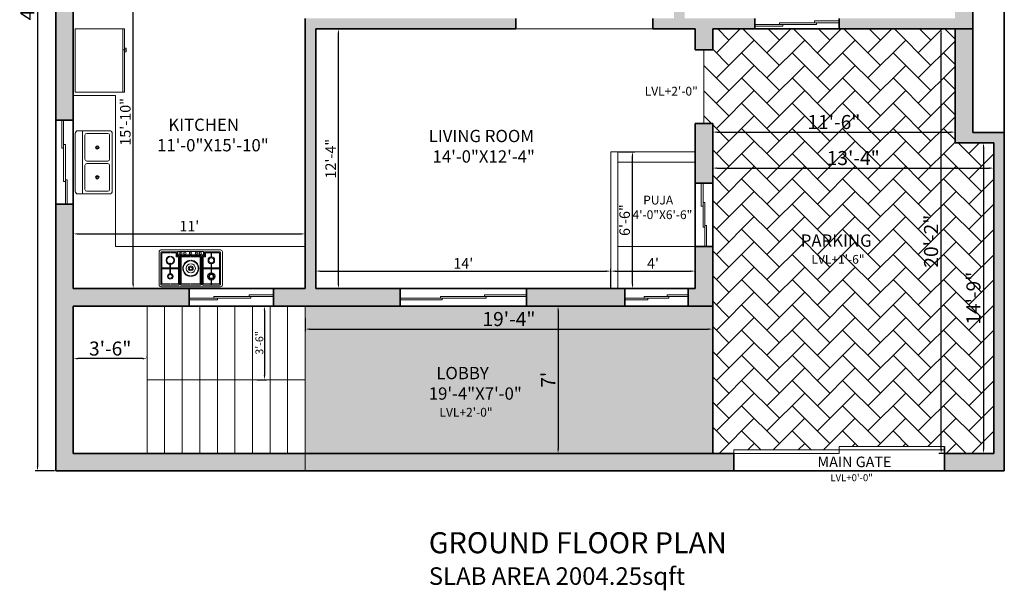
# Model space of a CAD drawing. Units: inches. Extents: x 3491 to 6898, y 1360 to 2019.
# Tile 6 of 9: x 5693 to 6254, y 1360 to 1686. Entities that reach past the tile are written whole.
import ezdxf

# ---------------------------------------------------------------- set-up
doc = ezdxf.new("R2010")
doc.units = ezdxf.units.IN
for name, color, linetype, lineweight in [('A-ANNO-DIMS', 2, 'Continuous', 18), ('A-ANNO-TEXT', 7, 'Continuous', 18), ('A-ANNO-TITL', 7, 'Continuous', 30), ('A-AREA-IDEN', 7, 'Continuous', 18), ('A-DOOR', 4, 'Continuous', 18), ('A-EQPM', 8, 'Continuous', 18), ('A-FLOR-CASE', 8, 'Continuous', 18), ('A-FLOR-FIXT', 8, 'Continuous', 18), ('A-FLOR-PATT', 252, 'Continuous', 13), ('A-FLOR-STRS', 7, 'Continuous', 18), ('A-GLAZ', 5, 'Continuous', 18), ('A-WALL', 7, 'Continuous', 35), ('A-WALL-PATT', 8, 'Continuous', 13)]:
    doc.layers.add(name, color=color, linetype=linetype, lineweight=lineweight)
doc.layers.add('A-WALL-OPEN', color=251, linetype='Continuous', lineweight=13, true_color=0x636466)
doc.styles.get("Standard").update_dxf_attribs({"font": 'arial.ttf'})
doc.dimstyles.new('ISO-25', dxfattribs={"dimtxt": 8, "dimasz": 2.5, "dimexe": 1.25, "dimexo": 0.625, "dimtad": 1, "dimdec": 1, "dimlunit": 3, "dimtxsty": 'Standard', "dimcen": 2.5, "dimclrt": 1, "dimadec": 0, "dimazin": 0, "dimtfac": 1, "dimtdec": 1, "dimtmove": 0, "dimatfit": 3, "dimfxl": 1, "dimarcsym": 0})

# ---------------------------------------------------------------- blocks, each defined once
blk = doc.blocks.new('*D53')
at = {"layer": 'A-ANNO-DIMS', "color": 0, "lineweight": -2, "transparency": 16777216}
for p, q in [((5712.99, 1972.37), (5701.98, 1972.37)), ((5703.23, 1969.87), (5703.23, 1430.87)), ((5712.99, 1428.37), (5701.98, 1428.37))]:
    blk.add_line(p, q, dxfattribs=at)
at = {"layer": 'A-ANNO-DIMS', "color": 0, "transparency": 16777216}
for points in [[(5702.81, 1969.87), (5703.65, 1969.87), (5703.23, 1972.37)], [(5702.81, 1430.87), (5703.65, 1430.87), (5703.23, 1428.37)]]:
    blk.add_solid(points, dxfattribs=at)
at = {"layer": 'Defpoints', "color": 0, "transparency": 16777216}
for p in [(5713.61, 1972.37), (5703.23, 1428.37), (5713.61, 1428.37)]:
    blk.add_point(p, dxfattribs=at)
at = {"layer": 'A-ANNO-DIMS', "color": 0, "transparency": 16777216, "insert": (5698.54, 1700.37), "char_height": 8, "attachment_point": 5, "rotation": 90}
blk.add_mtext('45\'-4"', dxfattribs=at)
blk = doc.blocks.new('*D49')
at = {"layer": 'A-ANNO-DIMS', "color": 0, "lineweight": -2, "transparency": 16777216}
for p, q in [((5723.61, 1493.03), (5723.61, 1493.65)), ((5763.11, 1492.4), (5726.11, 1492.4)), ((5765.61, 1493.03), (5765.61, 1493.65))]:
    blk.add_line(p, q, dxfattribs=at)
at = {"layer": 'A-ANNO-DIMS', "color": 0, "transparency": 16777216}
for points in [[(5726.11, 1492.82), (5726.11, 1491.99), (5723.61, 1492.4)], [(5763.11, 1492.82), (5763.11, 1491.99), (5765.61, 1492.4)]]:
    blk.add_solid(points, dxfattribs=at)
at = {"layer": 'Defpoints', "color": 0, "transparency": 16777216}
for p in [(5723.61, 1492.4), (5723.61, 1492.4), (5765.61, 1492.4)]:
    blk.add_point(p, dxfattribs=at)
at = {"layer": 'A-ANNO-DIMS', "color": 0, "transparency": 16777216, "insert": (5744.61, 1497.12), "char_height": 8, "attachment_point": 5}
blk.add_mtext('3\'-6"', dxfattribs=at)
blk = doc.blocks.new('*D31')
at = {"layer": 'A-ANNO-DIMS', "color": 0, "lineweight": -2, "transparency": 16777216}
for p, q in [((5828.32, 1522.37), (5833.67, 1522.37)), ((5832.42, 1519.87), (5832.42, 1482.87)), ((5828.32, 1480.37), (5833.67, 1480.37))]:
    blk.add_line(p, q, dxfattribs=at)
at = {"layer": 'A-ANNO-DIMS', "color": 0, "transparency": 16777216}
for points in [[(5832, 1519.87), (5832.83, 1519.87), (5832.42, 1522.37)], [(5832, 1482.87), (5832.83, 1482.87), (5832.42, 1480.37)]]:
    blk.add_solid(points, dxfattribs=at)
at = {"layer": 'Defpoints', "color": 0, "transparency": 16777216}
for p in [(5827.7, 1522.37), (5827.7, 1480.37), (5832.42, 1480.37)]:
    blk.add_point(p, dxfattribs=at)
at = {"layer": 'A-ANNO-DIMS', "color": 0, "transparency": 16777216, "insert": (5829.52, 1501.37), "char_height": 8, "attachment_point": 5, "rotation": 90}
blk.add_mtext('{\\H0.55556x;3\'-6"}', dxfattribs=at)
blk = doc.blocks.new('*D50')
at = {"layer": 'A-ANNO-DIMS', "color": 0, "lineweight": -2, "transparency": 16777216}
for p, q in [((5999.58, 1519.87), (5999.58, 1440.87)), ((6000.21, 1522.37), (6000.83, 1522.37)), ((6000.21, 1438.37), (6000.83, 1438.37))]:
    blk.add_line(p, q, dxfattribs=at)
at = {"layer": 'A-ANNO-DIMS', "color": 0, "transparency": 16777216}
for points in [[(5999.17, 1519.87), (6000, 1519.87), (5999.58, 1522.37)], [(5999.17, 1440.87), (6000, 1440.87), (5999.58, 1438.37)]]:
    blk.add_solid(points, dxfattribs=at)
at = {"layer": 'Defpoints', "color": 0, "transparency": 16777216}
for p in [(5999.58, 1522.37), (5999.58, 1438.37), (5999.58, 1438.37)]:
    blk.add_point(p, dxfattribs=at)
at = {"layer": 'A-ANNO-DIMS', "color": 0, "transparency": 16777216, "insert": (5994.96, 1480.37), "char_height": 8, "attachment_point": 5, "rotation": 90}
blk.add_mtext("7'", dxfattribs=at)
blk = doc.blocks.new('*D48')
at = {"layer": 'A-ANNO-DIMS', "color": 0, "lineweight": -2, "transparency": 16777216}
for p, q in [((6087.61, 1521.74), (6087.61, 1507.99)), ((5855.61, 1515.52), (5855.61, 1507.99)), ((5858.11, 1509.24), (6085.11, 1509.24))]:
    blk.add_line(p, q, dxfattribs=at)
at = {"layer": 'A-ANNO-DIMS', "color": 0, "transparency": 16777216}
for points in [[(5858.11, 1509.66), (5858.11, 1508.83), (5855.61, 1509.24)], [(6085.11, 1509.66), (6085.11, 1508.83), (6087.61, 1509.24)]]:
    blk.add_solid(points, dxfattribs=at)
at = {"layer": 'Defpoints', "color": 0, "transparency": 16777216}
for p in [(6087.61, 1522.37), (5855.61, 1516.15), (6087.61, 1509.24)]:
    blk.add_point(p, dxfattribs=at)
at = {"layer": 'A-ANNO-DIMS', "color": 0, "transparency": 16777216, "insert": (5971.61, 1513.95), "char_height": 8, "attachment_point": 5}
blk.add_mtext('19\'-4"', dxfattribs=at)
blk = doc.blocks.new('STOVE')
for p, q in [((11.85, 19.7), (11.55, 19.7)), ((11.55, 16.92), (11.55, 19.7)), ((11.85, 16.92), (11.55, 16.92)), ((11.85, 16.92), (11.85, 19.7)), ((-11.85, 13.73), (-11.85, 7.62)), ((-11.85, 13.73), (-11.55, 13.73)), ((-11.55, 13.73), (-11.55, 7.62)), ((11.85, 13.23), (11.55, 13.23)), ((11.55, 13.23), (11.55, 7.57)), ((11.85, 13.23), (11.85, 7.57)), ((-11.85, 10.75), (-16.4, 10.75)), ((-11.85, 10.25), (-16.4, 10.25)), ((-11.85, 7.62), (-11.55, 7.62)), ((-7, 10.75), (-11.55, 10.75)), ((-7, 10.25), (-11.55, 10.25)), ((7, 10.75), (11.55, 10.75)), ((7, 10.25), (11.55, 10.25)), ((11.85, 7.57), (11.55, 7.57)), ((11.85, 10.75), (16.4, 10.75)), ((11.85, 10.25), (16.4, 10.25)), ((-7, 3.9), (-8.4, 3.9)), ((-7.8, 3.3), (-7.8, 1)), ((-6.4, 3.3), (-7.8, 3.3)), ((7.3, 2.8), (-7.3, 2.8)), ((-7.3, 2.8), (-7.3, 0.8)), ((7.3, 0.8), (-7.3, 0.8)), ((-5.4, 3.9), (-6, 3.9)), ((-5.4, 3.9), (-0.15, 3.9)), ((0.15, 3.9), (5.4, 3.9)), ((6.4, 3.3), (7.8, 3.3)), ((7, 3.9), (8.4, 3.9)), ((7.3, 2.8), (7.3, 0.8)), ((7.8, 3.3), (7.8, 1)), ((8.4, 3.9), (8.4, 1.6)), ((11.85, 4.28), (11.55, 4.28)), ((11.55, 4.28), (11.55, 1.3)), ((11.85, 1.3), (11.55, 1.3)), ((11.85, 4.28), (11.85, 1.3))]:
    blk.add_line(p, q)
for points in [[(-17, 21), (17, 21, -0.414214), (18, 20), (18, 1, -0.414214), (17, 0), (-17, 0, -0.414214), (-18, 1), (-18, 20, -0.414214)], [(6, 3.3), (-6, 3.3), (-6, 19.4, -0.414214), (-5.4, 20), (5.4, 20, -0.414214), (6, 19.4)]]:
    blk.add_lwpolyline(points, format="xyb", close=True)
for points in [[(-7.8, 1), (-16.4, 1, -0.414214), (-17, 1.6), (-17, 19.4, -0.414214), (-16.4, 20), (-7, 20, -0.414214), (-6.4, 19.4), (-6.4, 3.3)], [(6.4, 19.4, -0.414214), (7, 20), (16.4, 20, -0.414214), (17, 19.4), (17, 1.6, -0.414214), (16.4, 1), (7.8, 1)]]:
    blk.add_lwpolyline(points, format="xyb")
for points in [[(-16.4, 15.22), (-16.4, 19.4), (-11.85, 19.4)], [(-11.55, 19.4), (-7, 19.4), (-7, 15.22)], [(-5.4, 15.22), (-5.4, 19.4), (-0.15, 19.4)], [(0.15, 19.4), (5.4, 19.4), (5.4, 15.22)], [(6.4, 3.3), (6.4, 19.4)], [(7, 15.22), (7, 19.4), (11.55, 19.4)], [(11.85, 19.4), (16.4, 19.4), (16.4, 15.22)], [(-16.4, 6.08), (-16.4, 14.92)], [(-7, 14.92), (-7, 6.08)], [(-5.4, 10.65), (-5.4, 14.92)], [(5.4, 14.92), (5.4, 10.65)], [(7, 6.08), (7, 14.92)], [(16.4, 14.92), (16.4, 6.08)], [(-11.85, 1.6), (-16.4, 1.6), (-16.4, 5.77)], [(-7, 5.77), (-7, 3.9)], [(-5.4, 6.08), (-5.4, 10.35)], [(-5.4, 3.9), (-5.4, 5.77)], [(5.4, 10.35), (5.4, 6.08)], [(5.4, 5.77), (5.4, 3.9)], [(7, 3.9), (7, 5.77)], [(16.4, 5.77), (16.4, 1.6), (11.85, 1.6)], [(-8.4, 3.9), (-8.4, 1.6), (-11.55, 1.6)], [(11.55, 1.6), (8.4, 1.6)]]:
    blk.add_lwpolyline(points)
for centre, radius in [((-11.7, 15.07), 1.1), ((0, 10.5), 1.4), ((0, 10.5), 0.8), ((11.7, 15.07), 1.6), ((11.7, 15.07), 1.1), ((11.7, 5.93), 1.4), ((-5.49, 1.8), 0.6), ((-3.3, 1.8), 0.6), ((0, 1.8), 0.6), ((3.39, 1.8), 0.6), ((5.57, 1.8), 0.6)]:
    blk.add_circle(centre, radius)
for centre, radius, start, end in [((11.7, 15.07), 2.1, 94.096, 175.904), ((11.7, 15.07), 2.1, 4.096, 85.904), ((-11.7, 15.07), 1.6, 95.3794, 174.6206), ((-11.7, 15.07), 1.6, 185.3794, 264.6206), ((-11.7, 15.07), 1.6, 5.3794, 84.6206), ((-11.7, 15.07), 1.6, 275.3794, 354.6206), ((0, 10.5), 4.6, 91.8687, 178.1313), ((0, 10.5), 4.3, 91.9991, 178.0009), ((0, 10.5), 2.6, 93.3074, 176.6926), ((0, 10.5), 4.6, 1.8687, 88.1313), ((0, 10.5), 4.3, 1.9991, 88.0009), ((0, 10.5), 2.6, 3.3074, 86.6926), ((11.7, 15.07), 2.1, 184.096, 265.904), ((11.7, 15.07), 2.1, 274.096, 355.904), ((-11.7, 5.93), 2.4, 93.5833, 176.4167), ((-11.7, 5.93), 2.4, 183.5833, 266.4167), ((-11.7, 5.93), 2, 94.3012, 175.6988), ((-11.7, 5.93), 2, 184.3012, 265.6988), ((-11.7, 5.93), 2.4, 3.5833, 86.4167), ((-11.7, 5.93), 2, 4.3012, 85.6988), ((-11.7, 5.93), 2.4, 273.5833, 356.4167), ((-11.7, 5.93), 2, 274.3012, 355.6988), ((0, 10.5), 4.6, 181.8687, 268.1313), ((0, 10.5), 4.3, 181.9991, 268.0009), ((0, 10.5), 2.6, 183.3074, 266.6926), ((0, 10.5), 4.6, 271.8687, 358.1313), ((0, 10.5), 4.3, 271.9991, 358.0009), ((0, 10.5), 2.6, 273.3074, 356.6926), ((11.7, 5.93), 1.9, 94.5281, 175.4719), ((11.7, 5.93), 1.9, 184.5281, 265.4719), ((11.7, 5.93), 1.9, 4.5281, 85.4719), ((11.7, 5.93), 1.9, 274.5281, 355.4719), ((-5.49, 1.8), 0.846, 89.9979, 270), ((-3.3, 1.8), 0.846, 89.9979, 270), ((0, 1.8), 0.846, 89.9979, 270), ((3.39, 1.8), 0.846, 89.9979, 270), ((5.57, 1.8), 0.846, 89.9979, 270)]:
    blk.add_arc(centre, radius, start, end)
blk = doc.blocks.new('Sink-double - 36 in top')
for p, q in [((-18, -4), (18, -4)), ((-0.75, -18.5), (-0.75, -6.5)), ((0.75, -6.5), (0.75, -18.5))]:
    blk.add_line(p, q)
for points in [[(-16.5, 0), (16.5, 0)], [(-18, -19.5), (-18, -1.5)], [(-15.5, -5.5), (-1.75, -5.5)], [(1.75, -5.5), (15.5, -5.5)], [(18, -1.5), (18, -19.5)], [(-16.5, -18.5), (-16.5, -6.5)], [(16.5, -6.5), (16.5, -18.5)], [(16.5, -21), (-16.5, -21)], [(-1.75, -19.5), (-15.5, -19.5)], [(15.5, -19.5), (1.75, -19.5)]]:
    blk.add_lwpolyline(points)
for centre, radius in [((-8.5, -12.5), 1), ((-8.5, -12.5), 0.5), ((8.5, -12.5), 1), ((8.5, -12.5), 0.5)]:
    blk.add_circle(centre, radius)
for centre, radius, start, end in [((-16.5, -1.5), 1.5, 90, 180), ((16.5, -1.5), 1.5, 0, 90), ((-15.5, -6.5), 1, 90, 180), ((-1.75, -6.5), 1, 0, 90), ((1.75, -6.5), 1, 90, 180), ((15.5, -6.5), 1, 0, 90), ((-16.5, -19.5), 1.5, 180, 270), ((-15.5, -18.5), 1, 180, 270), ((-1.75, -18.5), 1, 270, 0), ((1.75, -18.5), 1, 180, 270), ((15.5, -18.5), 1, 270, 0), ((16.5, -19.5), 1.5, 270, 0)]:
    blk.add_arc(centre, radius, start, end)
blk = doc.blocks.new('Refrigerator-2 door - 36 in top')
for p, q in [((0, -26.999999), (36, -26.999999)), ((11, -27.999999), (11, -28.999999)), ((12, -26.999999), (12, -28.999999)), ((13, -28.999999), (13, -27.999999)), ((11, -28.999999), (13, -28.999999))]:
    blk.add_line(p, q)
blk.add_lwpolyline([(0, -27.999999), (0, 0), (36, 0), (36, -27.999999)], close=True)
blk = doc.blocks.new('*D44')
at = {"layer": 'A-ANNO-DIMS', "color": 0, "lineweight": -2, "transparency": 16777216}
for p, q in [((6087.61, 1617.55), (6087.61, 1622.78)), ((6090.11, 1621.53), (6223.11, 1621.53)), ((6225.61, 1617.55), (6225.61, 1622.78))]:
    blk.add_line(p, q, dxfattribs=at)
at = {"layer": 'A-ANNO-DIMS', "color": 0, "transparency": 16777216}
for points in [[(6090.11, 1621.95), (6090.11, 1621.12), (6087.61, 1621.53)], [(6223.11, 1621.95), (6223.11, 1621.12), (6225.61, 1621.53)]]:
    blk.add_solid(points, dxfattribs=at)
at = {"layer": 'Defpoints', "color": 0, "transparency": 16777216}
for p in [(6225.61, 1621.53), (6087.61, 1616.92), (6225.61, 1616.92)]:
    blk.add_point(p, dxfattribs=at)
at = {"layer": 'A-ANNO-DIMS', "color": 0, "transparency": 16777216, "insert": (6156.61, 1626.24), "char_height": 8, "attachment_point": 5}
blk.add_mtext('11\'-6"', dxfattribs=at)
blk = doc.blocks.new('*D45')
at = {"layer": 'A-ANNO-DIMS', "color": 0, "lineweight": -2, "transparency": 16777216}
for p, q in [((6087.61, 1601.63), (6087.61, 1602.25)), ((6090.11, 1601), (6245.11, 1601)), ((6247.61, 1601.63), (6247.61, 1602.25))]:
    blk.add_line(p, q, dxfattribs=at)
at = {"layer": 'A-ANNO-DIMS', "color": 0, "transparency": 16777216}
for points in [[(6090.11, 1601.42), (6090.11, 1600.59), (6087.61, 1601)], [(6245.11, 1601.42), (6245.11, 1600.59), (6247.61, 1601)]]:
    blk.add_solid(points, dxfattribs=at)
at = {"layer": 'Defpoints', "color": 0, "transparency": 16777216}
for p in [(6087.61, 1601), (6247.61, 1601), (6247.61, 1601)]:
    blk.add_point(p, dxfattribs=at)
at = {"layer": 'A-ANNO-DIMS', "color": 0, "transparency": 16777216, "insert": (6167.61, 1605.72), "char_height": 8, "attachment_point": 5}
blk.add_mtext('13\'-4"', dxfattribs=at)
blk = doc.blocks.new('*D46')
at = {"layer": 'A-ANNO-DIMS', "color": 0, "lineweight": -2, "transparency": 16777216}
for p, q in [((6246.99, 1615.37), (6240.54, 1615.37)), ((6241.79, 1612.87), (6241.79, 1440.87)), ((6246.99, 1438.37), (6240.54, 1438.37))]:
    blk.add_line(p, q, dxfattribs=at)
at = {"layer": 'A-ANNO-DIMS', "color": 0, "transparency": 16777216}
for points in [[(6241.37, 1612.87), (6242.21, 1612.87), (6241.79, 1615.37)], [(6241.37, 1440.87), (6242.21, 1440.87), (6241.79, 1438.37)]]:
    blk.add_solid(points, dxfattribs=at)
at = {"layer": 'Defpoints', "color": 0, "transparency": 16777216}
for p in [(6247.61, 1615.37), (6241.79, 1438.37), (6247.61, 1438.37)]:
    blk.add_point(p, dxfattribs=at)
at = {"layer": 'A-ANNO-DIMS', "color": 0, "transparency": 16777216, "insert": (6237.08, 1526.87), "char_height": 8, "attachment_point": 5, "rotation": 90}
blk.add_mtext('14\'-9"', dxfattribs=at)
blk = doc.blocks.new('*D47')
at = {"layer": 'A-ANNO-DIMS', "color": 0, "lineweight": -2, "transparency": 16777216}
for p, q in [((6224.99, 1680.37), (6216.41, 1680.37)), ((6217.66, 1440.87), (6217.66, 1677.87)), ((6226.03, 1438.37), (6216.41, 1438.37))]:
    blk.add_line(p, q, dxfattribs=at)
at = {"layer": 'A-ANNO-DIMS', "color": 0, "transparency": 16777216}
for points in [[(6217.24, 1677.87), (6218.08, 1677.87), (6217.66, 1680.37)], [(6217.24, 1440.87), (6218.08, 1440.87), (6217.66, 1438.37)]]:
    blk.add_solid(points, dxfattribs=at)
at = {"layer": 'Defpoints', "color": 0, "transparency": 16777216}
for p in [(6217.66, 1680.37), (6225.61, 1680.37), (6226.65, 1438.37)]:
    blk.add_point(p, dxfattribs=at)
at = {"layer": 'A-ANNO-DIMS', "color": 0, "transparency": 16777216, "insert": (6212.95, 1559.37), "char_height": 8, "attachment_point": 5, "rotation": 90}
blk.add_mtext('20\'-2"', dxfattribs=at)
blk = doc.blocks.new('*D63')
at = {"layer": 'A-ANNO-DIMS', "color": 0, "lineweight": -2, "transparency": 16777216}
for p, q in [((5862.24, 1680.37), (5875.79, 1680.37)), ((5874.54, 1534.87), (5874.54, 1677.87)), ((5862.24, 1532.37), (5875.79, 1532.37))]:
    blk.add_line(p, q, dxfattribs=at)
at = {"layer": 'A-ANNO-DIMS', "color": 0, "transparency": 16777216}
for points in [[(5874.13, 1677.87), (5874.96, 1677.87), (5874.54, 1680.37)], [(5874.13, 1534.87), (5874.96, 1534.87), (5874.54, 1532.37)]]:
    blk.add_solid(points, dxfattribs=at)
at = {"layer": 'Defpoints', "color": 0, "transparency": 16777216}
for p in [(5861.61, 1680.37), (5874.54, 1680.37), (5861.61, 1532.37)]:
    blk.add_point(p, dxfattribs=at)
at = {"layer": 'A-ANNO-DIMS', "color": 0, "transparency": 16777216, "insert": (5870.91, 1606.37), "char_height": 6, "attachment_point": 5, "rotation": 90}
blk.add_mtext('12\'-4"', dxfattribs=at)
blk = doc.blocks.new('*D64')
at = {"layer": 'A-ANNO-DIMS', "color": 0, "lineweight": -2, "transparency": 16777216}
for p, q in [((5724.24, 1722.37), (5758.94, 1722.37)), ((5757.69, 1534.87), (5757.69, 1719.87)), ((5724.24, 1532.37), (5758.94, 1532.37))]:
    blk.add_line(p, q, dxfattribs=at)
at = {"layer": 'A-ANNO-DIMS', "color": 0, "transparency": 16777216}
for points in [[(5757.27, 1719.87), (5758.1, 1719.87), (5757.69, 1722.37)], [(5757.27, 1534.87), (5758.1, 1534.87), (5757.69, 1532.37)]]:
    blk.add_solid(points, dxfattribs=at)
at = {"layer": 'Defpoints', "color": 0, "transparency": 16777216}
for p in [(5723.61, 1722.37), (5757.69, 1722.37), (5723.61, 1532.37)]:
    blk.add_point(p, dxfattribs=at)
at = {"layer": 'A-ANNO-DIMS', "color": 0, "transparency": 16777216, "insert": (5754, 1627.37), "char_height": 6, "attachment_point": 5, "rotation": 90}
blk.add_mtext('15\'-10"', dxfattribs=at)
blk = doc.blocks.new('*D65')
at = {"layer": 'A-ANNO-DIMS', "color": 0, "lineweight": -2, "transparency": 16777216}
for p, q in [((5723.61, 1532.99), (5723.61, 1564.76)), ((5855.61, 1532.99), (5855.61, 1564.76)), ((5726.11, 1563.51), (5853.11, 1563.51))]:
    blk.add_line(p, q, dxfattribs=at)
at = {"layer": 'A-ANNO-DIMS', "color": 0, "transparency": 16777216}
for points in [[(5726.11, 1563.92), (5726.11, 1563.09), (5723.61, 1563.51)], [(5853.11, 1563.92), (5853.11, 1563.09), (5855.61, 1563.51)]]:
    blk.add_solid(points, dxfattribs=at)
at = {"layer": 'Defpoints', "color": 0, "transparency": 16777216}
for p in [(5855.61, 1563.51), (5723.61, 1532.37), (5855.61, 1532.37)]:
    blk.add_point(p, dxfattribs=at)
at = {"layer": 'A-ANNO-DIMS', "color": 0, "transparency": 16777216, "insert": (5789.61, 1567.15), "char_height": 6, "attachment_point": 5}
blk.add_mtext("11'", dxfattribs=at)
blk = doc.blocks.new('*D66')
at = {"layer": 'A-ANNO-DIMS', "color": 0, "lineweight": -2, "transparency": 16777216}
for p, q in [((5861.61, 1532.99), (5861.61, 1543.54)), ((5864.11, 1542.29), (6027.11, 1542.29)), ((6029.61, 1532.99), (6029.61, 1543.54))]:
    blk.add_line(p, q, dxfattribs=at)
at = {"layer": 'A-ANNO-DIMS', "color": 0, "transparency": 16777216}
for points in [[(5864.11, 1542.71), (5864.11, 1541.88), (5861.61, 1542.29)], [(6027.11, 1542.71), (6027.11, 1541.88), (6029.61, 1542.29)]]:
    blk.add_solid(points, dxfattribs=at)
at = {"layer": 'Defpoints', "color": 0, "transparency": 16777216}
for p in [(6029.61, 1542.29), (5861.61, 1532.37), (6029.61, 1532.37)]:
    blk.add_point(p, dxfattribs=at)
at = {"layer": 'A-ANNO-DIMS', "color": 0, "transparency": 16777216, "insert": (5945.61, 1545.93), "char_height": 6, "attachment_point": 5}
blk.add_mtext("14'", dxfattribs=at)
blk = doc.blocks.new('*D67')
at = {"layer": 'A-ANNO-DIMS', "color": 0, "lineweight": -2, "transparency": 16777216}
for p, q in [((6029.61, 1532.99), (6029.61, 1543.54)), ((6032.11, 1542.29), (6075.11, 1542.29)), ((6077.61, 1532.99), (6077.61, 1543.54))]:
    blk.add_line(p, q, dxfattribs=at)
at = {"layer": 'A-ANNO-DIMS', "color": 0, "transparency": 16777216}
for points in [[(6032.11, 1542.71), (6032.11, 1541.88), (6029.61, 1542.29)], [(6075.11, 1542.71), (6075.11, 1541.88), (6077.61, 1542.29)]]:
    blk.add_solid(points, dxfattribs=at)
at = {"layer": 'Defpoints', "color": 0, "transparency": 16777216}
for p in [(6077.61, 1542.29), (6029.61, 1532.37), (6077.61, 1532.37)]:
    blk.add_point(p, dxfattribs=at)
at = {"layer": 'A-ANNO-DIMS', "color": 0, "transparency": 16777216, "insert": (6053.61, 1545.92), "char_height": 6, "attachment_point": 5}
blk.add_mtext("4'", dxfattribs=at)
blk = doc.blocks.new('*D68')
at = {"layer": 'A-ANNO-DIMS', "color": 0, "lineweight": -2, "transparency": 16777216}
for p, q in [((6034.24, 1610.37), (6043.21, 1610.37)), ((6041.96, 1534.87), (6041.96, 1607.87)), ((6034.24, 1532.37), (6043.21, 1532.37))]:
    blk.add_line(p, q, dxfattribs=at)
at = {"layer": 'A-ANNO-DIMS', "color": 0, "transparency": 16777216}
for points in [[(6041.54, 1607.87), (6042.38, 1607.87), (6041.96, 1610.37)], [(6041.54, 1534.87), (6042.38, 1534.87), (6041.96, 1532.37)]]:
    blk.add_solid(points, dxfattribs=at)
at = {"layer": 'Defpoints', "color": 0, "transparency": 16777216}
for p in [(6033.61, 1610.37), (6041.96, 1610.37), (6033.61, 1532.37)]:
    blk.add_point(p, dxfattribs=at)
at = {"layer": 'A-ANNO-DIMS', "color": 0, "transparency": 16777216, "insert": (6038.27, 1571.37), "char_height": 6, "attachment_point": 5, "rotation": 90}
blk.add_mtext('6\'-6"', dxfattribs=at)
blk = doc.blocks.new('WIN-SLIDER-48IN')
for p, q in [((35, 1), (0, 1)), ((48, 2), (14, 2)), ((14, 2), (14, 1)), ((16, 1), (16, 0)), ((34, 3), (34, 2)), ((48, 3), (34, 3)), ((35, 2), (35, 1)), ((16, 0), (0, 0))]:
    blk.add_line(p, q)
blk = doc.blocks.new('WIN-SLIDER-36IN')
for p, q in [((25, 1), (0, 1)), ((13, 0), (0, 0)), ((36, 2), (11, 2)), ((11, 2), (11, 1)), ((13, 1), (13, 0)), ((24, 3), (24, 2)), ((36, 3), (24, 3)), ((25, 2), (25, 1))]:
    blk.add_line(p, q)
blk = doc.blocks.new('WIN-SLIDER-72IN')
for p, q in [((0, 1), (49, 1)), ((0, 0), (23.95, 0)), ((22.95, 2), (72, 2)), ((22.95, 1), (22.95, 2)), ((23.95, 0), (23.95, 1)), ((48, 3), (72, 3)), ((48, 2), (48, 3)), ((49, 1), (49, 2))]:
    blk.add_line(p, q)
blk = doc.blocks.new('STAIR-RETURN-FLIGHT')
for p, q in [((0, 84), (0, 0)), ((10, 84), (10, 0)), ((20, 84), (20, 0)), ((30, 84), (30, 0)), ((40, 84), (40, 0)), ((50, 84), (50, 0)), ((60, 84), (60, 0)), ((70, 84), (70, 0)), ((80, 84), (80, 0)), ((0, 42), (90, 42))]:
    blk.add_line(p, q)
blk = doc.blocks.new('COUNTER-KITCHEN-L')
for p, q in [((24, 86.04), (0, 86.04)), ((24, 86.04), (24, 0)), ((132, 0), (24, 0))]:
    blk.add_line(p, q)
blk = doc.blocks.new('PUJA-ALCOVE-48X78')
for p, q in [((0, 78), (0, 0)), ((48, 78), (0, 78)), ((4, 78), (4, 0)), ((48, 72), (4, 72)), ((48, 24), (4, 24))]:
    blk.add_line(p, q)

msp = doc.modelspace()

# ---------------------------------------------------------------- hatches: boundary and pattern name
at = {"layer": 'A-FLOR-PATT'}
h = msp.add_hatch(dxfattribs=at)
h.set_pattern_fill('AR-HBONE', color=256, scale=0.1)
h.set_pattern_definition([(45, (2181.48, 0), (0, 14.36841), [30.48, -10.16]), (135, (2188.664, 7.184), (1e-15, 14.36841), [30.48, -10.16])])
h.paths.add_polyline_path([(6219.61, 1442.37), (6219.61, 1438.37), (6247.61, 1438.37), (6247.61, 1615.37), (6225.61, 1615.37), (6225.61, 1680.37), (6087.61, 1680.37), (6087.61, 1668.37), (6082.61, 1668.37), (6082.61, 1626.37), (6087.61, 1626.37), (6087.61, 1438.37), (6099.61, 1438.37), (6099.61, 1440.37), (6159.61, 1440.37), (6159.61, 1442.37)])
h.paths.add_polyline_path([(6140.03, 1617.93), (6172.5, 1617.93), (6172.5, 1634.41), (6140.03, 1634.41)], flags=24)
h.paths.add_polyline_path([(6151.03, 1597.4), (6183.5, 1597.4), (6183.5, 1613.89), (6151.03, 1613.89)], flags=24)
h.paths.add_polyline_path([(6245.4, 1510.28), (6245.4, 1542.75), (6228.91, 1542.75), (6228.91, 1510.28)], flags=24)
h.paths.add_polyline_path([(6221.27, 1543.23), (6221.27, 1575.7), (6204.78, 1575.7), (6204.78, 1543.23)], flags=24)
h.paths.add_polyline_path([(6135.23, 1543.14), (6182.75, 1543.14), (6182.75, 1566.66), (6135.23, 1566.66)], flags=24)
h = msp.add_hatch(dxfattribs=at)
h.set_pattern_fill('ANSI36', color=256, scale=0.5, angle=45)
h.set_pattern_definition([(90, (2181.4796, 0), (-1.5875, 2.778125), [3.96875, -0.79375, 0, -0.79375])])
h.paths.add_polyline_path([(5855.61, 1438.37), (6087.61, 1438.37), (6087.61, 1522.37), (5855.61, 1522.37)])
h.paths.add_polyline_path([(6003.33, 1474.19), (6003.33, 1486.54), (5986.84, 1486.54), (5986.84, 1474.19)], flags=24)
h.paths.add_polyline_path([(5955.03, 1505.64), (5987.5, 1505.64), (5987.5, 1522.12), (5955.03, 1522.12)], flags=24)
h.paths.add_polyline_path([(5923.15, 1455.94), (5977.56, 1455.94), (5977.56, 1491.16), (5923.15, 1491.16)], flags=24)
at = {"layer": 'A-WALL-PATT'}
h = msp.add_hatch(color=256, dxfattribs=at)
h.dxf.hatch_style = 1
h.paths.add_polyline_path([(6037.61, 1532.37), (5981.61, 1532.37), (5981.61, 1522.37), (6037.61, 1522.37)])
h.paths.add_polyline_path([(6087.61, 1626.37), (6077.61, 1626.37), (6077.61, 1592.37), (6087.61, 1592.37)])
h.paths.add_polyline_path([(6087.61, 1556.37), (6077.61, 1556.37), (6077.61, 1532.37), (6073.61, 1532.37), (6073.61, 1522.37), (6087.61, 1522.37)])
h.paths.add_polyline_path([(5909.61, 1532.37), (5861.61, 1532.37), (5861.61, 1680.37), (5975.61, 1680.37), (5975.61, 1686.37), (5855.61, 1686.37), (5855.61, 1532.37), (5837.64, 1532.37), (5837.64, 1522.37), (5909.61, 1522.37)])
h.paths.add_polyline_path([(5789.64, 1532.37), (5723.61, 1532.37), (5723.61, 1580.4), (5713.61, 1580.4), (5713.61, 1428.37), (5855.61, 1428.37), (5855.61, 1438.37), (5723.61, 1438.37), (5723.61, 1522.37), (5789.64, 1522.37)])
h.paths.add_polyline_path([(5723.61, 1722.37), (5801.61, 1722.37), (5801.61, 1782.37), (5795.61, 1782.37), (5795.61, 1728.37), (5723.61, 1728.37), (5723.61, 1770.37), (5713.61, 1770.37), (5713.61, 1628.4), (5723.61, 1628.4)])
h.paths.add_polyline_path([(6087.61, 1680.37), (6111.61, 1680.37), (6111.61, 1686.37), (6071.61, 1686.37), (6071.61, 1776.37), (6065.61, 1776.37), (6065.61, 1686.37), (6053.61, 1686.37), (6053.61, 1680.37), (6077.61, 1680.37), (6077.61, 1668.37), (6087.61, 1668.37)])
h.paths.add_polyline_path([(6235.61, 1719.37), (6225.61, 1719.37), (6225.61, 1686.37), (6159.61, 1686.37), (6159.61, 1680.37), (6235.61, 1680.37)])
h.paths.add_polyline_path([(6235.61, 1857.37), (6225.61, 1857.37), (6225.61, 1818.37), (6065.61, 1818.37), (6065.61, 1812.37), (6225.61, 1812.37), (6225.61, 1779.37), (6235.61, 1779.37)])
h.paths.add_polyline_path([(6029.61, 1872.37), (6023.61, 1872.37), (6023.61, 1818.37), (5963.61, 1818.37), (5963.61, 1902.37), (5981.61, 1902.37), (5981.61, 1908.37), (5939.61, 1908.37), (5939.61, 1902.37), (5957.61, 1902.37), (5957.61, 1818.37), (5897.61, 1818.37), (5897.61, 1872.37), (5891.61, 1872.37), (5891.61, 1812.37), (6029.61, 1812.37)])
h.paths.add_polyline_path([(5723.61, 1857.37), (5713.61, 1857.37), (5713.61, 1794.37), (5723.61, 1794.37), (5723.61, 1812.37), (5855.61, 1812.37), (5855.61, 1818.37), (5723.61, 1818.37)])
h.paths.add_polyline_path([(5723.61, 1962.37), (5891.61, 1962.37), (5891.61, 1938.37), (5897.61, 1938.37), (5897.61, 1962.37), (6023.61, 1962.37), (6023.61, 1938.37), (6029.61, 1938.37), (6029.61, 1962.37), (6225.61, 1962.37), (6225.61, 1923.37), (6235.61, 1923.37), (6235.61, 1972.37), (5713.61, 1972.37), (5713.61, 1923.37), (5723.61, 1923.37)])
h.paths.add_polyline_path([(5915.61, 1908.37), (5891.61, 1908.37), (5891.61, 1902.37), (5915.61, 1902.37)])
h.paths.add_polyline_path([(6029.61, 1908.37), (6005.61, 1908.37), (6005.61, 1902.37), (6029.61, 1902.37)], flags=17)
h = msp.add_hatch(color=256, dxfattribs=at)
h.dxf.hatch_style = 1
h.paths.add_polyline_path([(6099.61, 1438.37), (5855.61, 1438.37), (5855.61, 1428.37), (6099.61, 1428.37)])
h.paths.add_polyline_path([(6253.61, 1621.37), (6235.61, 1621.37), (6235.61, 1680.37), (6225.61, 1680.37), (6225.61, 1615.37), (6247.61, 1615.37), (6247.61, 1438.37), (6219.61, 1438.37), (6219.61, 1428.37), (6253.61, 1428.37)])

# ---------------------------------------------------------------- linework, layer by layer
at = {"layer": 'A-DOOR'}
for p, q in [((6082.61, 1626.37), (6082.61, 1668.37)), ((6159.61, 1438.37), (6159.61, 1442.37)), ((6159.61, 1442.37), (6219.61, 1442.37)), ((6219.61, 1440.37), (6099.61, 1440.37)), ((6099.61, 1440.37), (6099.61, 1438.37)), ((6159.61, 1438.37), (6099.61, 1438.37))]:
    msp.add_line(p, q, dxfattribs=at)
at = {"layer": 'A-FLOR-STRS'}
msp.add_line((5855.61, 1522.37), (5855.61, 1428.37), dxfattribs=at)
at = {"layer": 'A-WALL'}
for p, q in [((5713.61, 1972.37), (5713.61, 1428.37)), ((6235.61, 1972.37), (6235.61, 1621.37)), ((6253.61, 1428.37), (6253.61, 1972.37)), ((5723.61, 1722.37), (5723.61, 1532.37)), ((5855.61, 1686.37), (5855.61, 1532.37)), ((5975.61, 1686.37), (5975.61, 1680.37)), ((6053.61, 1686.37), (6053.61, 1680.37)), ((6111.61, 1686.37), (6111.61, 1680.37)), ((6159.61, 1686.37), (6159.61, 1680.37)), ((5975.61, 1680.37), (5861.61, 1680.37)), ((5861.61, 1680.37), (5861.61, 1532.37)), ((6077.61, 1680.37), (6053.61, 1680.37)), ((6077.61, 1680.37), (6077.61, 1668.37)), ((6235.61, 1680.37), (6087.61, 1680.37)), ((6087.61, 1680.37), (6087.61, 1668.37)), ((6225.61, 1680.37), (6225.61, 1615.37)), ((6087.61, 1668.37), (6077.61, 1668.37)), ((5723.61, 1628.4), (5713.61, 1628.4)), ((6087.61, 1626.37), (6077.61, 1626.37)), ((6077.61, 1626.37), (6077.61, 1532.37)), ((6087.61, 1626.37), (6087.61, 1438.37)), ((6253.61, 1621.37), (6235.61, 1621.37)), ((6247.61, 1615.37), (6225.61, 1615.37)), ((6247.61, 1438.37), (6247.61, 1615.37)), ((6087.61, 1592.37), (6077.61, 1592.37)), ((5723.61, 1580.4), (5713.61, 1580.4)), ((6087.61, 1556.37), (6077.61, 1556.37)), ((5855.61, 1532.37), (5723.61, 1532.37)), ((5789.64, 1532.37), (5789.64, 1522.37)), ((5837.64, 1532.37), (5837.64, 1522.37)), ((6077.61, 1532.37), (5861.61, 1532.37)), ((5909.61, 1522.37), (5909.61, 1532.37)), ((5981.61, 1522.37), (5981.61, 1532.37)), ((6037.61, 1532.37), (6037.61, 1522.37)), ((6073.61, 1532.37), (6073.61, 1522.37)), ((6087.61, 1522.37), (5723.61, 1522.37)), ((5723.61, 1522.37), (5723.61, 1438.37)), ((6219.61, 1442.37), (6219.61, 1428.37)), ((5723.61, 1438.37), (6099.61, 1438.37)), ((6099.61, 1438.37), (6099.61, 1428.37)), ((6219.61, 1438.37), (6247.61, 1438.37)), ((5713.61, 1428.37), (6253.61, 1428.37))]:
    msp.add_line(p, q, dxfattribs=at)
at = {"layer": 'A-WALL-OPEN'}
msp.add_line((5975.61, 1680.37), (6053.61, 1680.37), dxfattribs=at)

# ---------------------------------------------------------------- block references
at = {"layer": 'A-EQPM', "xscale": -1}
for name, p, rotation in [('Refrigerator-2 door - 36 in top', (5724.76, 1680.37), 90), ('STOVE', (5790.48, 1554.37), 180)]:
    msp.add_blockref(name, p, dxfattribs=dict(at, rotation=rotation))
at = {"layer": 'A-FLOR-CASE'}
for name, p in [('COUNTER-KITCHEN-L', (5723.61, 1556.37)), ('PUJA-ALCOVE-48X78', (6029.61, 1532.37))]:
    msp.add_blockref(name, p, dxfattribs=at)
at = {"layer": 'A-FLOR-FIXT', "rotation": 90}
msp.add_blockref('Sink-double - 36 in top', (5724.76, 1604.3), dxfattribs=at)
at = {"layer": 'A-FLOR-STRS'}
msp.add_blockref('STAIR-RETURN-FLIGHT', (5765.61, 1438.37), dxfattribs=at)
at = {"layer": 'A-GLAZ'}
for name, p in [('WIN-SLIDER-48IN', (6111.61, 1681.87)), ('WIN-SLIDER-48IN', (5789.64, 1525.87)), ('WIN-SLIDER-72IN', (5909.61, 1525.87)), ('WIN-SLIDER-36IN', (6037.61, 1525.87))]:
    msp.add_blockref(name, p, dxfattribs=at)
at = {"layer": 'A-GLAZ', "rotation": 270}
for name, p in [('WIN-SLIDER-48IN', (5717.11, 1628.4)), ('WIN-SLIDER-36IN', (6081.11, 1592.37))]:
    msp.add_blockref(name, p, dxfattribs=at)

# ---------------------------------------------------------------- texts
at = {"layer": 'A-ANNO-TEXT', "attachment_point": 1}
for s, width, insert, char_height in [('{LVL+2\'-0"}', 33.0959, (6048.92, 1647.35), 5), ('{\\H0.85714x;MAIN GATE}\\P{\\H0.57143x;      LVL+0\'-0"}', 121.6144, (6147.26, 1436.56), 7)]:
    msp.add_mtext_dynamic_manual_height_columns(s, width=width, gutter_width=12.5, heights=[0], dxfattribs=dict(at, insert=insert, char_height=char_height))
at = {"layer": 'A-ANNO-TITL', "insert": (5925.97, 1393.48), "char_height": 12, "attachment_point": 1}
msp.add_mtext_dynamic_manual_height_columns('GROUND FLOOR PLAN\\P{\\H0.83333x;SLAB AREA 2004.25sqft}', width=285.9409, gutter_width=12.5, heights=[0], dxfattribs=at)
at = {"layer": 'A-AREA-IDEN', "attachment_point": 1}
for s, width, insert, char_height in [('   KITCHEN\\P11\'-0"X15\'-10"', 86.9528, (5771.28, 1629.22), 7), ('LIVING ROOM\\P 14\'-0"X12\'-4"', 121.6144, (5925.97, 1622.81), 7), ('    PUJA\\P4\'-0"X6\'-6"', 33.0959, (6041.96, 1585.28), 5), ('PARKING\\P{\\H0.71429x;    LVL+1\'-6"}', 121.6144, (6137.74, 1563.18), 7), ('  LOBBY\\P19\'-4"X7\'-0"\\P{\\H0.71429x;    LVL+2\'-0"}', 121.6144, (5925.97, 1487.68), 7)]:
    msp.add_mtext_dynamic_manual_height_columns(s, width=width, gutter_width=12.5, heights=[0], dxfattribs=dict(at, insert=insert, char_height=char_height))

# ---------------------------------------------------------------- dimensions: what is measured, and where the dimension line sits
at = {"layer": 'A-ANNO-DIMS'}
for base, p1, p2, angle, override, picture, middle in [((5703.23, 1428.37), (5713.61, 1972.37), (5713.61, 1428.37), 90, {"dimclrd": 0, "dimclre": 0, "dimclrt": 0}, '*D53', (5698.54, 1700.37)), ((5757.69, 1722.37), (5723.61, 1532.37), (5723.61, 1722.37), 270, {"dimtxt": 6, "dimclrd": 0, "dimclre": 0, "dimclrt": 0}, '*D64', (5754, 1627.37)), ((5874.54, 1680.37), (5861.61, 1532.37), (5861.61, 1680.37), 270, {"dimtxt": 6, "dimclrd": 0, "dimclre": 0, "dimclrt": 0}, '*D63', (5870.91, 1606.37)), ((6217.66, 1680.37), (6226.65, 1438.37), (6225.61, 1680.37), 90, {"dimclrd": 0, "dimclre": 0, "dimclrt": 0}, '*D47', (6212.95, 1559.37)), ((6241.79, 1438.37), (6247.61, 1615.37), (6247.61, 1438.37), 90, {"dimclrd": 0, "dimclre": 0, "dimclrt": 0}, '*D46', (6237.08, 1526.87)), ((6041.96, 1610.37), (6033.61, 1532.37), (6033.61, 1610.37), 90, {"dimtxt": 6, "dimclrd": 0, "dimclre": 0, "dimclrt": 0}, '*D68', (6038.27, 1571.37)), ((5999.58, 1438.37), (5999.58, 1522.37), (5999.58, 1438.37), 90, {"dimclrd": 0, "dimclre": 0, "dimclrt": 0}, '*D50', (5994.96, 1480.37))]:
    dim = msp.add_linear_dim(base=base, p1=p1, p2=p2, angle=angle, dimstyle='ISO-25', override=override, dxfattribs=at)
    dim.commit()
    dim.dimension.update_dxf_attribs({"geometry": picture, "text_midpoint": middle})
for base, p1, p2, override, picture, middle in [((6225.61, 1621.53), (6087.61, 1616.92), (6225.61, 1616.92), {"dimclrd": 0, "dimclre": 0, "dimclrt": 0}, '*D44', (6156.61, 1626.24)), ((6247.61, 1601), (6087.61, 1601), (6247.61, 1601), {"dimclrd": 0, "dimclre": 0, "dimclrt": 0}, '*D45', (6167.61, 1605.72)), ((5855.61, 1563.51), (5723.61, 1532.37), (5855.61, 1532.37), {"dimtxt": 6, "dimclrd": 0, "dimclre": 0, "dimclrt": 0}, '*D65', (5789.61, 1567.15)), ((6029.61, 1542.29), (5861.61, 1532.37), (6029.61, 1532.37), {"dimtxt": 6, "dimclrd": 0, "dimclre": 0, "dimclrt": 0}, '*D66', (5945.61, 1545.93)), ((6077.61, 1542.29), (6029.61, 1532.37), (6077.61, 1532.37), {"dimtxt": 6, "dimclrd": 0, "dimclre": 0, "dimclrt": 0, "dimtmove": 1}, '*D67', (6053.61, 1545.92)), ((6087.61, 1509.24), (5855.61, 1516.15), (6087.61, 1522.37), {"dimclrd": 0, "dimclre": 0, "dimclrt": 0}, '*D48', (5971.61, 1513.95)), ((5723.61, 1492.4), (5765.61, 1492.4), (5723.61, 1492.4), {"dimclrd": 0, "dimclre": 0, "dimclrt": 0}, '*D49', (5744.61, 1497.12))]:
    dim = msp.add_linear_dim(base=base, p1=p1, p2=p2, dimstyle='ISO-25', override=override, dxfattribs=at)
    dim.commit()
    dim.dimension.update_dxf_attribs({"geometry": picture, "text_midpoint": middle})
dim = msp.add_linear_dim(base=(5832.42, 1480.37), p1=(5827.7, 1522.37), p2=(5827.7, 1480.37), angle=90, text='{\\H0.55556x;<>}', dimstyle='ISO-25', override={"dimclrd": 0, "dimclre": 0, "dimclrt": 0}, dxfattribs=at)
dim.commit()
dim.dimension.update_dxf_attribs({"geometry": '*D31', "text_midpoint": (5829.52, 1501.37)})

doc.saveas('drawing.dxf')
